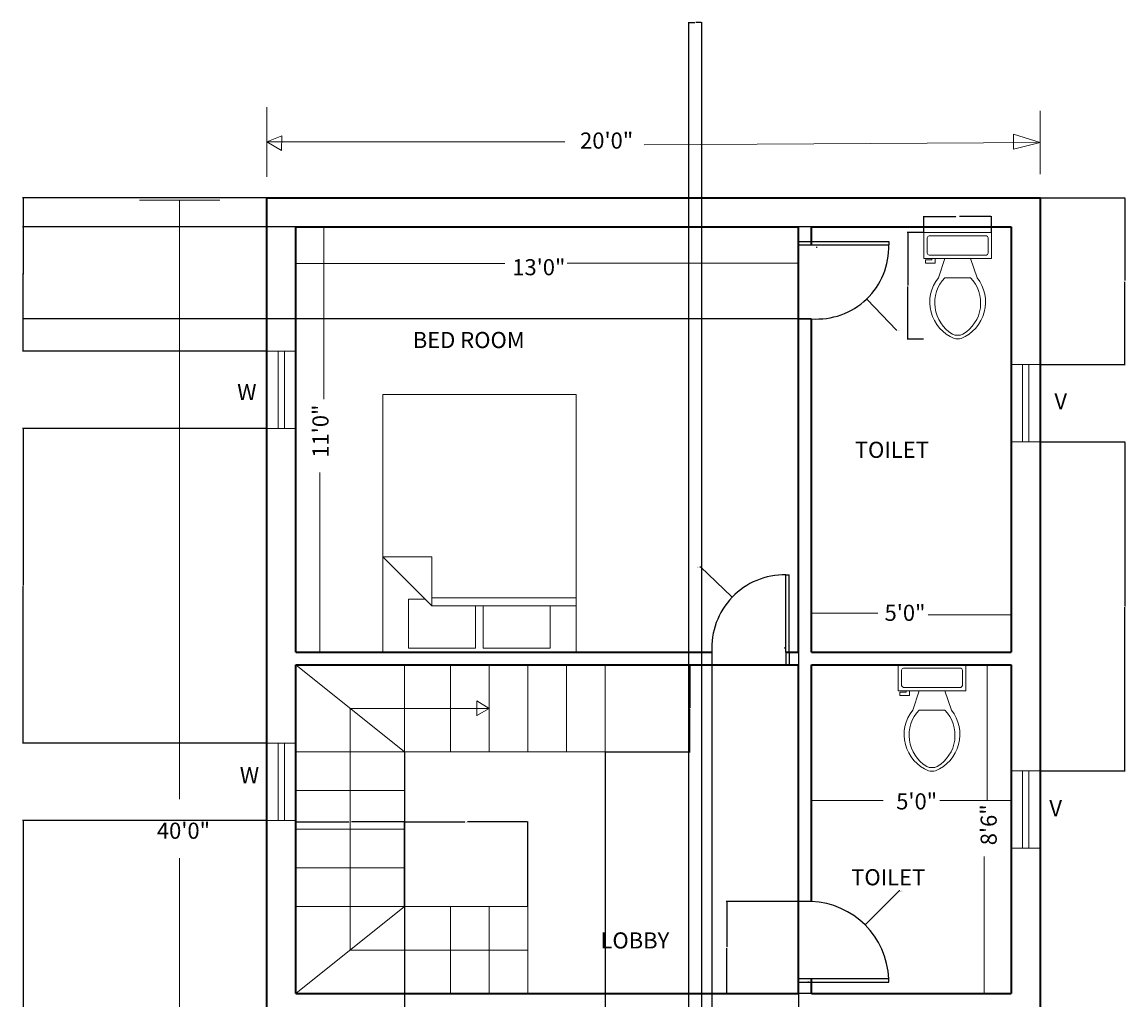
# Model space of a CAD drawing. Units: inches. Extents: x -58 to 719, y -488 to 73.
# Tile 2 of 3: x -58 to 284, y -231 to 73. Entities that reach past the tile are written whole.
import ezdxf

# ---------------------------------------------------------------- set-up
doc = ezdxf.new("R2010")
doc.units = ezdxf.units.IN
doc.header["$MEASUREMENT"] = 0
for name, color, linetype, lineweight in [('A-ANNO-DIMS', 2, 'Continuous', 13), ('A-ANNO-TEXT', 7, 'Continuous', 18), ('A-AREA-IDEN', 7, 'Continuous', 25), ('A-DOOR', 3, 'Continuous', 25), ('A-FLOR-FIXT', 9, 'Continuous', 18), ('A-FLOR-STRS', 7, 'Continuous', 18), ('A-FURN', 8, 'Continuous', 18), ('A-GLAZ', 4, 'Continuous', 18), ('A-WALL', 7, 'Continuous', 35)]:
    doc.layers.add(name, color=color, linetype=linetype, lineweight=lineweight)
doc.styles.get("Standard").update_dxf_attribs({"font": 'arial.ttf'})
doc.dimstyles.get("Standard").update_dxf_attribs({"dimtxt": 0.18, "dimasz": 0.18, "dimexe": 0.18, "dimexo": 0.0625, "dimgap": 0.09, "dimtad": 0, "dimtih": 1, "dimtoh": 1, "dimdec": 4, "dimzin": 0, "dimdsep": 46, "dimtxsty": 'Standard', "dimcen": 0.09, "dimadec": 0, "dimazin": 0, "dimtfac": 1, "dimtdec": 4, "dimtofl": 0, "dimtmove": 0, "dimatfit": 3, "dimfxl": 1, "dimtolj": 1, "dimtzin": 0, "dimarcsym": 0})

# ---------------------------------------------------------------- blocks, each defined once
blk = doc.blocks.new('Bed - Queen')
for p, q in [((0, -80.00003), (0, 0)), ((0, 0), (59.99999, 0)), ((59.99999, 0), (59.99999, -80.00003)), ((7.99999, -1.2), (28.79998, -1.2)), ((7.99999, -14.4), (7.99999, -1.2)), ((28.79998, -1.2), (28.79998, -14.4)), ((31.19999, -1.2), (51.99999, -1.2)), ((31.19999, -14.4), (31.19999, -1.2)), ((51.99999, -1.2), (51.99999, -16.4)), ((0, -14.4), (44.8, -14.4)), ((44.8, -16.8), (0, -16.8)), ((59.99999, -29.6), (44.8, -14.4)), ((44.8, -14.4), (44.8, -29.6)), ((51.99999, -16.4), (46.79936, -16.4)), ((44.8, -29.6), (59.99999, -29.6)), ((59.99999, -80.00003), (0, -80.00003))]:
    blk.add_line(p, q)
blk = doc.blocks.new('Toilet - top')
for p, q in [((9.5, -6), (9.5, -2)), ((-10, -8.5), (-8, -8.5)), ((-10, -9.5), (-10, -8.5)), ((-7, -9.5), (-10, -9.5)), ((-8, -8.5), (-8, -8)), ((-7, -8), (-7, -9.5)), ((-4, -8), (-6, -14)), ((4, -8), (6, -14)), ((4, -14), (-4, -14))]:
    blk.add_line(p, q)
blk.add_lwpolyline([(10.5, -8), (10.5, 0), (-10.5, 0), (-10.5, -8)], close=True)
for points in [[(-9.5, -2), (-9.5, -6)], [(8.5, -1), (-8.5, -1)], [(-8.5, -7), (8.5, -7)]]:
    blk.add_lwpolyline(points)
for centre, radius, start, end in [((-8.62, -1.88), 0.884, 81.8699, 188.1301), ((8.62, -1.88), 0.884, 351.8699, 98.1301), ((-8.62, -6.12), 0.884, 171.8699, 278.1301), ((8.62, -6.12), 0.884, 261.8699, 8.1301), ((3.52, -21.58), 12.17, 141.4691, 247.9714), ((4.2, -21.82), 11.33, 136.3677, 238.9468), ((-3.52, -21.58), 12.17, 292.0284, 38.5307), ((-4.2, -21.82), 11.33, 301.053, 43.6321), ((0, -27.88), 4, 245.7318, 294.2682), ((0, -29), 4, 254.8605, 285.1395)]:
    blk.add_arc(centre, radius, start, end)
blk = doc.blocks.new('WIN-24IN')
for p, q in [((3.5, 24), (3.5, 0)), ((5.5, 24), (5.5, 0))]:
    blk.add_line(p, q)
blk.add_lwpolyline([(0, 24), (9, 24), (9, 0), (0, 0)], close=True)
blk = doc.blocks.new('VENT-24IN')
for p, q in [((3.5, 24), (3.5, 0)), ((5.5, 24), (5.5, 0))]:
    blk.add_line(p, q)
blk.add_lwpolyline([(0, 24), (9, 24), (9, 0), (0, 0)], close=True)
blk = doc.blocks.new('*D13')
at = {"layer": 'A-ANNO-DIMS', "color": 0, "lineweight": -2, "transparency": 16777216}
for p, q in [((221.46, 7.7), (216.39, 7.7)), ((216.57, 7.52), (216.57, -8.64)), ((216.57, -25.17), (216.57, -9.01)), ((221.46, -25.35), (216.39, -25.35))]:
    blk.add_line(p, q, dxfattribs=at)
at = {"layer": 'A-ANNO-DIMS', "color": 0, "transparency": 16777216}
for points in [[(216.54, 7.52), (216.6, 7.52), (216.57, 7.7)], [(216.54, -25.17), (216.6, -25.17), (216.57, -25.35)]]:
    blk.add_solid(points, dxfattribs=at)
at = {"layer": 'Defpoints', "color": 0, "transparency": 16777216}
for p in [(216.57, 7.7), (221.53, 7.7), (221.53, -25.35)]:
    blk.add_point(p, dxfattribs=at)
at = {"layer": 'A-ANNO-DIMS', "color": 0, "transparency": 16777216, "insert": (216.57, -8.83), "char_height": 0.18, "attachment_point": 5}
blk.add_mtext('\\A1;WC 33 TYP.', dxfattribs=at)
blk = doc.blocks.new('*D14')
at = {"layer": 'A-ANNO-DIMS', "color": 0, "lineweight": -2, "transparency": 16777216}
for p, q in [((221.53, 7.76), (221.53, 12.83)), ((221.71, 12.65), (231.5, 12.65)), ((242.35, 12.65), (232.56, 12.65)), ((242.53, 7.76), (242.53, 12.83))]:
    blk.add_line(p, q, dxfattribs=at)
at = {"layer": 'A-ANNO-DIMS', "color": 0, "transparency": 16777216}
for points in [[(221.71, 12.68), (221.71, 12.62), (221.53, 12.65)], [(242.35, 12.68), (242.35, 12.62), (242.53, 12.65)]]:
    blk.add_solid(points, dxfattribs=at)
at = {"layer": 'Defpoints', "color": 0, "transparency": 16777216}
for p in [(242.53, 12.65), (221.53, 7.7), (242.53, 7.7)]:
    blk.add_point(p, dxfattribs=at)
at = {"layer": 'A-ANNO-DIMS', "color": 0, "transparency": 16777216, "insert": (232.03, 12.65), "char_height": 0.18, "attachment_point": 5}
blk.add_mtext('\\A1;21 TYP.', dxfattribs=at)
blk = doc.blocks.new('*D28')
at = {"layer": 'A-ANNO-DIMS', "color": 0, "lineweight": -2, "transparency": 16777216}
for p, q in [((17.55, 18.48), (-58.2, 18.48)), ((-58.02, 18.3), (-58.02, -5.15)), ((-58.02, -28.97), (-58.02, -5.52)), ((17.55, -29.15), (-58.2, -29.15))]:
    blk.add_line(p, q, dxfattribs=at)
at = {"layer": 'A-ANNO-DIMS', "color": 0, "transparency": 16777216}
for points in [[(-58.05, 18.3), (-57.99, 18.3), (-58.02, 18.48)], [(-58.05, -28.97), (-57.99, -28.97), (-58.02, -29.15)]]:
    blk.add_solid(points, dxfattribs=at)
at = {"layer": 'Defpoints', "color": 0, "transparency": 16777216}
for p in [(17.61, 18.48), (-58.02, -29.15), (17.61, -29.15)]:
    blk.add_point(p, dxfattribs=at)
at = {"layer": 'A-ANNO-DIMS', "color": 0, "transparency": 16777216, "insert": (-58.02, -5.34), "char_height": 0.18, "attachment_point": 5}
blk.add_mtext('\\A1;47.63', dxfattribs=at)
blk = doc.blocks.new('*D29')
at = {"layer": 'A-ANNO-DIMS', "color": 0, "lineweight": -2, "transparency": 16777216}
for p, q in [((17.55, -53.15), (-58.2, -53.15)), ((-58.02, -53.33), (-58.02, -101.81)), ((-58.02, -150.65), (-58.02, -102.17)), ((17.55, -150.83), (-58.2, -150.83))]:
    blk.add_line(p, q, dxfattribs=at)
at = {"layer": 'A-ANNO-DIMS', "color": 0, "transparency": 16777216}
for points in [[(-58.05, -53.33), (-57.99, -53.33), (-58.02, -53.15)], [(-58.05, -150.65), (-57.99, -150.65), (-58.02, -150.83)]]:
    blk.add_solid(points, dxfattribs=at)
at = {"layer": 'Defpoints', "color": 0, "transparency": 16777216}
for p in [(17.61, -53.15), (-58.02, -150.83), (17.61, -150.83)]:
    blk.add_point(p, dxfattribs=at)
at = {"layer": 'A-ANNO-DIMS', "color": 0, "transparency": 16777216, "insert": (-58.02, -101.99), "char_height": 0.18, "attachment_point": 5}
blk.add_mtext('\\A1;97.68', dxfattribs=at)
blk = doc.blocks.new('*D30')
at = {"layer": 'A-ANNO-DIMS', "color": 0, "lineweight": -2, "transparency": 16777216}
for p, q in [((17.55, -174.83), (-58.2, -174.83)), ((-58.02, -175.01), (-58.02, -256.1)), ((-58.02, -337.55), (-58.02, -256.46)), ((17.55, -337.73), (-58.2, -337.73))]:
    blk.add_line(p, q, dxfattribs=at)
at = {"layer": 'A-ANNO-DIMS', "color": 0, "transparency": 16777216}
for points in [[(-58.05, -175.01), (-57.99, -175.01), (-58.02, -174.83)], [(-58.05, -337.55), (-57.99, -337.55), (-58.02, -337.73)]]:
    blk.add_solid(points, dxfattribs=at)
at = {"layer": 'Defpoints', "color": 0, "transparency": 16777216}
for p in [(17.61, -174.83), (-58.02, -337.73), (17.61, -337.73)]:
    blk.add_point(p, dxfattribs=at)
at = {"layer": 'A-ANNO-DIMS', "color": 0, "transparency": 16777216, "insert": (-58.02, -256.28), "char_height": 0.18, "attachment_point": 5}
blk.add_mtext('\\A1;162.9', dxfattribs=at)
blk = doc.blocks.new('*D31')
at = {"layer": 'A-ANNO-DIMS', "color": 0, "lineweight": -2, "transparency": 16777216}
for p, q in [((257.67, 18.48), (284.04, 18.48)), ((283.86, 18.3), (283.86, -7.21)), ((283.86, -33.08), (283.86, -7.57)), ((257.67, -33.26), (284.04, -33.26))]:
    blk.add_line(p, q, dxfattribs=at)
at = {"layer": 'A-ANNO-DIMS', "color": 0, "transparency": 16777216}
for points in [[(283.83, 18.3), (283.89, 18.3), (283.86, 18.48)], [(283.83, -33.08), (283.89, -33.08), (283.86, -33.26)]]:
    blk.add_solid(points, dxfattribs=at)
at = {"layer": 'Defpoints', "color": 0, "transparency": 16777216}
for p in [(257.61, 18.48), (257.61, -33.26), (283.86, -33.26)]:
    blk.add_point(p, dxfattribs=at)
at = {"layer": 'A-ANNO-DIMS', "color": 0, "transparency": 16777216, "insert": (283.86, -7.39), "char_height": 0.18, "attachment_point": 5}
blk.add_mtext('\\A1;51.74', dxfattribs=at)
blk = doc.blocks.new('*D32')
at = {"layer": 'A-ANNO-DIMS', "color": 0, "lineweight": -2, "transparency": 16777216}
for p, q in [((257.67, -57.26), (284.04, -57.26)), ((283.86, -57.44), (283.86, -108.16)), ((283.86, -159.24), (283.86, -108.52)), ((257.67, -159.42), (284.04, -159.42))]:
    blk.add_line(p, q, dxfattribs=at)
at = {"layer": 'A-ANNO-DIMS', "color": 0, "transparency": 16777216}
for points in [[(283.83, -57.44), (283.89, -57.44), (283.86, -57.26)], [(283.83, -159.24), (283.89, -159.24), (283.86, -159.42)]]:
    blk.add_solid(points, dxfattribs=at)
at = {"layer": 'Defpoints', "color": 0, "transparency": 16777216}
for p in [(257.61, -57.26), (257.61, -159.42), (283.86, -159.42)]:
    blk.add_point(p, dxfattribs=at)
at = {"layer": 'A-ANNO-DIMS', "color": 0, "transparency": 16777216, "insert": (283.86, -108.34), "char_height": 0.18, "attachment_point": 5}
blk.add_mtext('\\A1;102.16', dxfattribs=at)
blk = doc.blocks.new('*D41')
at = {"layer": 'A-ANNO-DIMS', "color": 0, "lineweight": -2, "transparency": 16777216}
for p, q in [((26.61, -201.46), (26.61, -175.09)), ((26.79, -175.27), (43.1, -175.27)), ((60.2, -175.27), (43.89, -175.27)), ((60.38, -201.46), (60.38, -175.09))]:
    blk.add_line(p, q, dxfattribs=at)
at = {"layer": 'A-ANNO-DIMS', "color": 0, "transparency": 16777216}
for points in [[(26.79, -175.24), (26.79, -175.3), (26.61, -175.27)], [(60.2, -175.24), (60.2, -175.3), (60.38, -175.27)]]:
    blk.add_solid(points, dxfattribs=at)
at = {"layer": 'Defpoints', "color": 0, "transparency": 16777216}
for p in [(60.38, -175.27), (26.61, -201.52), (60.38, -201.52)]:
    blk.add_point(p, dxfattribs=at)
at = {"layer": 'A-ANNO-DIMS', "color": 0, "transparency": 16777216, "insert": (43.5, -175.27), "char_height": 0.18, "attachment_point": 5}
blk.add_mtext('\\A1;33.77', dxfattribs=at)
blk = doc.blocks.new('*D42')
at = {"layer": 'A-ANNO-DIMS', "color": 0, "lineweight": -2, "transparency": 16777216}
for p, q in [((122.67, -126.52), (149.04, -126.52)), ((148.86, -126.7), (148.86, -139.84)), ((148.86, -153.34), (148.86, -140.2)), ((122.67, -153.52), (149.04, -153.52))]:
    blk.add_line(p, q, dxfattribs=at)
at = {"layer": 'A-ANNO-DIMS', "color": 0, "transparency": 16777216}
for points in [[(148.83, -126.7), (148.89, -126.7), (148.86, -126.52)], [(148.83, -153.34), (148.89, -153.34), (148.86, -153.52)]]:
    blk.add_solid(points, dxfattribs=at)
at = {"layer": 'Defpoints', "color": 0, "transparency": 16777216}
for p in [(122.61, -126.52), (122.61, -153.52), (148.86, -153.52)]:
    blk.add_point(p, dxfattribs=at)
at = {"layer": 'A-ANNO-DIMS', "color": 0, "transparency": 16777216, "insert": (148.86, -140.02), "char_height": 0.18, "attachment_point": 5}
blk.add_mtext('\\A1;27', dxfattribs=at)
blk = doc.blocks.new('*D43')
at = {"layer": 'A-ANNO-DIMS', "color": 0, "lineweight": -2, "transparency": 16777216}
for p, q in [((60.38, -153.59), (60.38, -487.95)), ((122.61, -153.59), (122.61, -487.95)), ((60.56, -487.77), (91.1, -487.77)), ((122.43, -487.77), (91.89, -487.77))]:
    blk.add_line(p, q, dxfattribs=at)
at = {"layer": 'A-ANNO-DIMS', "color": 0, "transparency": 16777216}
for points in [[(60.56, -487.74), (60.56, -487.8), (60.38, -487.77)], [(122.43, -487.74), (122.43, -487.8), (122.61, -487.77)]]:
    blk.add_solid(points, dxfattribs=at)
at = {"layer": 'Defpoints', "color": 0, "transparency": 16777216}
for p in [(60.38, -153.52), (122.61, -153.52), (122.61, -487.77)]:
    blk.add_point(p, dxfattribs=at)
at = {"layer": 'A-ANNO-DIMS', "color": 0, "transparency": 16777216, "insert": (91.5, -487.77), "char_height": 0.18, "attachment_point": 5}
blk.add_mtext('\\A1;62.23', dxfattribs=at)
blk = doc.blocks.new('*D44')
at = {"layer": 'A-ANNO-DIMS', "color": 0, "lineweight": -2, "transparency": 16777216}
for p, q in [((60.38, -201.46), (60.38, -175.09)), ((60.56, -175.27), (79.1, -175.27)), ((98.43, -175.27), (79.89, -175.27)), ((98.61, -201.46), (98.61, -175.09))]:
    blk.add_line(p, q, dxfattribs=at)
at = {"layer": 'A-ANNO-DIMS', "color": 0, "transparency": 16777216}
for points in [[(60.56, -175.24), (60.56, -175.3), (60.38, -175.27)], [(98.43, -175.24), (98.43, -175.3), (98.61, -175.27)]]:
    blk.add_solid(points, dxfattribs=at)
at = {"layer": 'Defpoints', "color": 0, "transparency": 16777216}
for p in [(98.61, -175.27), (60.38, -201.52), (98.61, -201.52)]:
    blk.add_point(p, dxfattribs=at)
at = {"layer": 'A-ANNO-DIMS', "color": 0, "transparency": 16777216, "insert": (79.5, -175.27), "char_height": 0.18, "attachment_point": 5}
blk.add_mtext('\\A1;38.23', dxfattribs=at)
blk = doc.blocks.new('*D49')
at = {"layer": 'A-ANNO-DIMS', "color": 0, "lineweight": -2, "transparency": 16777216}
for p, q in [((155.75, -122.59), (155.75, -487.95)), ((182.61, -122.59), (182.61, -487.95)), ((155.93, -487.77), (168.71, -487.77)), ((182.43, -487.77), (169.64, -487.77))]:
    blk.add_line(p, q, dxfattribs=at)
at = {"layer": 'A-ANNO-DIMS', "color": 0, "transparency": 16777216}
for points in [[(155.93, -487.74), (155.93, -487.8), (155.75, -487.77)], [(182.43, -487.74), (182.43, -487.8), (182.61, -487.77)]]:
    blk.add_solid(points, dxfattribs=at)
at = {"layer": 'Defpoints', "color": 0, "transparency": 16777216}
for p in [(155.75, -122.52), (182.61, -122.52), (182.61, -487.77)]:
    blk.add_point(p, dxfattribs=at)
at = {"layer": 'A-ANNO-DIMS', "color": 0, "transparency": 16777216, "insert": (169.18, -487.77), "char_height": 0.18, "attachment_point": 5}
blk.add_mtext('\\A1;26.867', dxfattribs=at)
blk = doc.blocks.new('*D50')
at = {"layer": 'A-ANNO-DIMS', "color": 0, "lineweight": -2, "transparency": 16777216}
for p, q in [((186.55, 9.48), (-58.2, 9.48)), ((-58.02, 9.3), (-58.02, -4.61)), ((-58.02, -18.88), (-58.02, -4.98)), ((186.55, -19.06), (-58.2, -19.06))]:
    blk.add_line(p, q, dxfattribs=at)
at = {"layer": 'A-ANNO-DIMS', "color": 0, "transparency": 16777216}
for points in [[(-58.05, 9.3), (-57.99, 9.3), (-58.02, 9.48)], [(-58.05, -18.88), (-57.99, -18.88), (-58.02, -19.06)]]:
    blk.add_solid(points, dxfattribs=at)
at = {"layer": 'Defpoints', "color": 0, "transparency": 16777216}
for p in [(186.61, 9.48), (-58.02, -19.06), (186.61, -19.06)]:
    blk.add_point(p, dxfattribs=at)
at = {"layer": 'A-ANNO-DIMS', "color": 0, "transparency": 16777216, "insert": (-58.02, -4.79), "char_height": 0.18, "attachment_point": 5}
blk.add_mtext('\\A1;28.54', dxfattribs=at)
blk = doc.blocks.new('*D51')
at = {"layer": 'A-ANNO-DIMS', "color": 0, "lineweight": -2, "transparency": 16777216}
for p, q in [((186.55, -199.98), (160.18, -199.98)), ((160.36, -200.16), (160.36, -214.07)), ((160.36, -228.34), (160.36, -214.43)), ((186.55, -228.52), (160.18, -228.52))]:
    blk.add_line(p, q, dxfattribs=at)
at = {"layer": 'A-ANNO-DIMS', "color": 0, "transparency": 16777216}
for points in [[(160.33, -200.16), (160.39, -200.16), (160.36, -199.98)], [(160.33, -228.34), (160.39, -228.34), (160.36, -228.52)]]:
    blk.add_solid(points, dxfattribs=at)
at = {"layer": 'Defpoints', "color": 0, "transparency": 16777216}
for p in [(160.36, -199.98), (186.61, -199.98), (186.61, -228.52)]:
    blk.add_point(p, dxfattribs=at)
at = {"layer": 'A-ANNO-DIMS', "color": 0, "transparency": 16777216, "insert": (160.36, -214.25), "char_height": 0.18, "attachment_point": 5}
blk.add_mtext('\\A1;28.54', dxfattribs=at)
blk = doc.blocks.new('*D57')
at = {"layer": 'A-ANNO-DIMS', "color": 0, "lineweight": -2, "transparency": 16777216}
for p, q in [((148.61, -377.52), (148.61, 73.06)), ((148.79, 72.88), (150.46, 72.88)), ((152.43, 72.88), (150.76, 72.88)), ((152.61, -377.52), (152.61, 73.06))]:
    blk.add_line(p, q, dxfattribs=at)
at = {"layer": 'A-ANNO-DIMS', "color": 0, "transparency": 16777216}
for points in [[(148.79, 72.91), (148.79, 72.85), (148.61, 72.88)], [(152.43, 72.91), (152.43, 72.85), (152.61, 72.88)]]:
    blk.add_solid(points, dxfattribs=at)
at = {"layer": 'Defpoints', "color": 0, "transparency": 16777216}
for p in [(152.61, 72.88), (148.61, -377.58), (152.61, -377.58)]:
    blk.add_point(p, dxfattribs=at)
at = {"layer": 'A-ANNO-DIMS', "color": 0, "transparency": 16777216, "insert": (150.61, 72.88), "char_height": 0.18, "attachment_point": 5}
blk.add_mtext('\\A1;4', dxfattribs=at)
blk = doc.blocks.new('*D60')
at = {"layer": 'A-ANNO-DIMS', "color": 0, "lineweight": -2, "transparency": 16777216}
for p, q in [((152, -96.09), (152.18, -96.09)), ((152.18, -96.09), (161.89, -105.39)), ((178.33, -121.23), (178.51, -121.23)), ((178.42, -121.32), (178.42, -121.14))]:
    blk.add_line(p, q, dxfattribs=at)
at = {"layer": 'A-ANNO-DIMS', "color": 0, "transparency": 16777216}
blk.add_solid([(161.91, -105.37), (161.87, -105.41), (162.02, -105.52)], dxfattribs=at)
at = {"layer": 'Defpoints', "color": 0, "transparency": 16777216}
for p in [(162.02, -105.52), (178.42, -121.23)]:
    blk.add_point(p, dxfattribs=at)
at = {"layer": 'A-ANNO-DIMS', "color": 0, "transparency": 16777216, "insert": (151.54, -96.09), "char_height": 0.18, "attachment_point": 5}
blk.add_mtext('\\A1;R22.71', dxfattribs=at)
blk = doc.blocks.new('*D61')
at = {"layer": 'A-ANNO-DIMS', "color": 0, "lineweight": -2, "transparency": 16777216}
for p, q in [((188.26, 3.14), (188.44, 3.14)), ((188.35, 3.05), (188.35, 3.23)), ((213.01, -22.59), (203.89, -13.07)), ((213.19, -22.59), (213.01, -22.59))]:
    blk.add_line(p, q, dxfattribs=at)
at = {"layer": 'A-ANNO-DIMS', "color": 0, "transparency": 16777216}
blk.add_solid([(203.91, -13.05), (203.87, -13.09), (203.77, -12.94)], dxfattribs=at)
at = {"layer": 'Defpoints', "color": 0, "transparency": 16777216}
for p in [(188.35, 3.14), (203.77, -12.94)]:
    blk.add_point(p, dxfattribs=at)
at = {"layer": 'A-ANNO-DIMS', "color": 0, "transparency": 16777216, "insert": (213.74, -22.59), "char_height": 0.18, "attachment_point": 5}
blk.add_mtext('\\A1;R22.273', dxfattribs=at)
blk = doc.blocks.new('*D62')
at = {"layer": 'A-ANNO-DIMS', "color": 0, "lineweight": -2, "transparency": 16777216}
for p, q in [((213.9, -196.7), (203.46, -207.13)), ((214.08, -196.7), (213.9, -196.7)), ((185.65, -224.86), (185.83, -224.86)), ((185.74, -224.95), (185.74, -224.77))]:
    blk.add_line(p, q, dxfattribs=at)
at = {"layer": 'A-ANNO-DIMS', "color": 0, "transparency": 16777216}
blk.add_solid([(203.44, -207.11), (203.49, -207.15), (203.34, -207.26)], dxfattribs=at)
at = {"layer": 'Defpoints', "color": 0, "transparency": 16777216}
for p in [(203.34, -207.26), (185.74, -224.86)]:
    blk.add_point(p, dxfattribs=at)
at = {"layer": 'A-ANNO-DIMS', "color": 0, "transparency": 16777216, "insert": (214.56, -196.7), "char_height": 0.18, "attachment_point": 5}
blk.add_mtext('\\A1;R24.89', dxfattribs=at)

msp = doc.modelspace()

# ---------------------------------------------------------------- linework, layer by layer
at = {"layer": 'A-ANNO-DIMS'}
for p, q in [((17.6125, 25.0283), (17.6125, 46.6293)), ((257.6125, 25.8138), (257.6125, 45.4511)), ((22.2716, 37.7231), (17.6125, 35.8288)), ((22.2315, 33.162), (22.2716, 37.7231)), ((249.366, 38.2807), (249.366, 33.5899)), ((257.6125, 35.6324), (249.366, 38.2807)), ((17.6125, 35.8288), (110.1276, 35.8288)), ((17.6125, 35.8288), (22.2315, 33.162)), ((134.7642, 34.9502), (257.6125, 35.6324)), ((249.366, 33.5899), (257.6125, 35.6324)), ((3.0105, 17.8018), (-21.9117, 17.8018)), ((-9.4506, 17.8018), (-9.4506, -151.1187)), ((35.2818, 9.477), (35.2818, -43.9909)), ((26.6125, -1.9438), (91.5244, -1.9438)), ((110.8063, -1.8001), (182.6125, -1.8001)), ((34.1307, -66.8274), (34.1307, -122.523)), ((207.2932, -110.4277), (186.6125, -110.4277)), ((222.8264, -111.0077), (248.6125, -111.0077)), ((241.1751, -168.631), (241.1751, -126.523)), ((-9.4506, -151.1187), (-9.4506, -168.1887)), ((208.8765, -168.631), (186.6125, -168.631)), ((226.472, -168.631), (248.6125, -168.631)), ((-9.4506, -208.4652), (-9.4506, -186.5319)), ((240.211, -185.9652), (240.211, -228.523)), ((-9.4506, -208.4652), (-9.4506, -461.523))]:
    msp.add_line(p, q, dxfattribs=at)
at = {"layer": 'A-DOOR'}
for p, q in [((182.6125, 4.9358), (186.6125, 4.9358)), ((182.6125, 3.9358), (186.6125, 3.9358)), ((186.6125, 4.9358), (210.6125, 4.9358)), ((186.6125, 3.9358), (210.6125, 3.9358)), ((210.6125, 4.9358), (210.6125, 3.9358)), ((182.6125, -19.0642), (186.6125, -19.0642)), ((178.7455, -122.523), (178.7455, -98.523)), ((178.7455, -98.523), (179.7455, -98.523)), ((179.7455, -122.523), (179.7455, -98.523)), ((155.7455, -122.523), (155.7455, -126.523)), ((178.7455, -122.523), (178.7455, -126.523)), ((179.7455, -122.523), (179.7455, -126.523)), ((186.6125, -199.9829), (182.6125, -199.9829)), ((210.6125, -223.9829), (182.6125, -223.9829)), ((182.6125, -224.9829), (186.6125, -224.9829)), ((186.6125, -224.9829), (210.6125, -224.9829)), ((210.6125, -224.9829), (210.6125, -223.9829))]:
    msp.add_line(p, q, dxfattribs=at)
for centre, radius, start, end in [((188.3542, 3.1401), 22.2725, 265.5149, 2.047349), ((178.42, -121.2319), 22.7112, 89.17876, 183.25899), ((185.7369, -224.8584), 24.891, 2.01582, 87.98418)]:
    msp.add_arc(centre, radius, start, end, dxfattribs=at)
at = {"layer": 'A-FLOR-STRS'}
for p, q in [((26.6125, -126.523), (60.3821, -153.523)), ((60.3821, -126.523), (60.3821, -228.523)), ((74.6125, -153.523), (74.6125, -126.523)), ((86.6125, -153.523), (86.6125, -126.523)), ((98.6125, -153.523), (98.6125, -126.523)), ((110.6125, -153.523), (110.6125, -126.523)), ((122.6125, -153.523), (122.6125, -126.523)), ((43.4973, -215.023), (43.4973, -140.023)), ((43.4973, -140.023), (86.6125, -140.023)), ((82.8428, -137.6838), (82.8428, -142.2823)), ((82.8428, -137.6838), (86.6125, -140.023)), ((86.6125, -140.023), (82.8428, -142.1994)), ((122.6125, -153.523), (26.6125, -153.523)), ((60.3821, -165.523), (26.6125, -165.523)), ((60.3821, -177.523), (26.6125, -177.523)), ((60.3821, -189.523), (26.6125, -189.523)), ((98.6125, -201.523), (26.6125, -201.523)), ((26.6125, -228.523), (60.3821, -201.523)), ((74.6125, -228.523), (74.6125, -201.523)), ((86.6125, -228.523), (86.6125, -201.523)), ((98.6125, -228.523), (98.6125, -201.523)), ((98.6125, -215.023), (43.4973, -215.023))]:
    msp.add_line(p, q, dxfattribs=at)
at = {"layer": 'A-WALL'}
for p, q in [((26.6125, 9.477), (182.6125, 9.477)), ((26.6125, -122.523), (26.6125, 9.477)), ((182.6125, -122.523), (182.6125, 9.477)), ((186.6125, 9.477), (248.6125, 9.477)), ((186.6125, 3.9358), (186.6125, 9.477)), ((248.6125, 9.477), (248.6125, -122.523)), ((186.6125, -122.523), (186.6125, -19.0642)), ((26.6125, -122.523), (155.7455, -122.523)), ((178.7455, -122.523), (182.6125, -122.523)), ((186.6125, -122.523), (248.6125, -122.523)), ((26.6125, -126.523), (182.6125, -126.523)), ((26.6125, -228.523), (26.6125, -126.523)), ((182.6125, -228.523), (182.6125, -126.523)), ((186.6125, -126.523), (248.6125, -126.523)), ((186.6125, -199.9829), (186.6125, -126.523)), ((248.6125, -126.523), (248.6125, -228.523)), ((186.6125, -228.523), (186.6125, -223.9829)), ((26.6125, -228.523), (182.6125, -228.523)), ((186.6125, -228.523), (248.6125, -228.523))]:
    msp.add_line(p, q, dxfattribs=at)
msp.add_lwpolyline([(17.6125, 18.477), (257.6125, 18.477), (257.6125, -461.523), (17.6125, -461.523)], close=True, dxfattribs=at)

# ---------------------------------------------------------------- block references
at = {"layer": 'A-FLOR-FIXT'}
for p in [(232.0273, 7.6958), (224.0617, -126.523)]:
    msp.add_blockref('Toilet - top', p, dxfattribs=at)
at = {"layer": 'A-FURN', "rotation": 180}
msp.add_blockref('Bed - Queen', (113.5937, -122.523), dxfattribs=at)
at = {"layer": 'A-GLAZ'}
for name, p in [('WIN-24IN', (17.612, -53.15)), ('VENT-24IN', (248.612, -57.262)), ('WIN-24IN', (17.612, -174.8327)), ('VENT-24IN', (248.612, -183.419))]:
    msp.add_blockref(name, p, dxfattribs=at)

# ---------------------------------------------------------------- texts
at = {"layer": 'A-ANNO-DIMS', "char_height": 5, "attachment_point": 1}
for s, width, insert in [('20\'0"', 28.703953, (114.8461, 38.7744)), ('13\'0"', 29.490631, (93.7994, -0.5447)), ('5\'0"', 18.491526, (209.3359, -107.8433)), ('5\'0"', 25.867981, (212.953, -166.3822)), ('40\'0"', 31.98226, (-16.4861, -175.484))]:
    msp.add_mtext_dynamic_manual_height_columns(s, width=width, gutter_width=25, heights=[0], dxfattribs=dict(at, insert=insert))
at = {"layer": 'A-ANNO-DIMS', "char_height": 5, "attachment_point": 1, "rotation": 90}
for s, width, insert in [('11\'0"', 10.973264, (31.782, -62.1803)), ('8\'6"', 12.173174, (239.1427, -182.507))]:
    msp.add_mtext_dynamic_manual_height_columns(s, width=width, gutter_width=25, heights=[0], dxfattribs=dict(at, insert=insert))
at = {"layer": 'A-ANNO-TEXT', "char_height": 5, "attachment_point": 1}
for s, width, insert in [('W', 17.81108, (8.4361, -39.3163)), ('V', 10.767555, (262.0349, -42.1619)), ('W', 14.30611, (9.2437, -158.2478)), ('V', 11.337096, (260.4655, -168.4838))]:
    msp.add_mtext_dynamic_manual_height_columns(s, width=width, gutter_width=25, heights=[0], dxfattribs=dict(at, insert=insert))
at = {"layer": 'A-AREA-IDEN', "char_height": 5, "attachment_point": 1}
for s, width, insert in [('BED ROOM', 52.122972, (62.9371, -23.1505)), ('TOILET', 36.88469, (200.1267, -57.2357)), ('TOILET', 33.856624, (198.9865, -189.9401)), ('LOBBY', 41.464849, (121.1802, -209.5542))]:
    msp.add_mtext_dynamic_manual_height_columns(s, width=width, gutter_width=25, heights=[0], dxfattribs=dict(at, insert=insert))

# ---------------------------------------------------------------- dimensions: what is measured, and where the dimension line sits
at = {"layer": 'A-ANNO-DIMS'}
for base, p1, p2, override, picture, middle in [((152.6125, 72.8793), (148.6125, -377.5847), (152.6125, -377.5847), {"dimdec": 0, "dimlfac": 1, "dimrnd": 0, "dimzin": 0, "dimdsep": 46, "dimlunit": 2}, '*D57', (150.6125, 72.8793)), ((182.6125, -487.773), (155.7455, -122.523), (182.6125, -122.523), {"dimdec": 3, "dimlfac": 1, "dimrnd": 0, "dimzin": 0, "dimdsep": 46, "dimlunit": 2}, '*D49', (169.179, -487.773)), ((122.6125, -487.773), (60.3821, -153.523), (122.6125, -153.523), {"dimdec": 2, "dimlfac": 1, "dimrnd": 0, "dimzin": 0, "dimdsep": 46, "dimlunit": 2}, '*D43', (91.4973, -487.773)), ((60.3821, -175.273), (26.6125, -201.523), (60.3821, -201.523), {"dimdec": 2, "dimlfac": 1, "dimrnd": 0, "dimzin": 0, "dimdsep": 46, "dimlunit": 2}, '*D41', (43.4973, -175.273)), ((98.6125, -175.273), (60.3821, -201.523), (98.6125, -201.523), {"dimdec": 2, "dimlfac": 1, "dimrnd": 0, "dimzin": 0, "dimdsep": 46, "dimlunit": 2}, '*D44', (79.4973, -175.273))]:
    dim = msp.add_linear_dim(base=base, p1=p1, p2=p2, dimstyle='Standard', override=override, dxfattribs=at)
    dim.commit()
    dim.dimension.update_dxf_attribs({"geometry": picture, "text_midpoint": middle})
for base, p1, p2, angle, override, picture, middle in [((-58.0187, -29.15), (17.6125, 18.477), (17.6125, -29.15), 90, {"dimdec": 2, "dimlfac": 1, "dimrnd": 0, "dimzin": 0, "dimdsep": 46, "dimlunit": 2}, '*D28', (-58.0187, -5.3365)), ((283.8625, -33.2617), (257.6125, 18.477), (257.6125, -33.2617), 90, {"dimdec": 2, "dimlfac": 1, "dimrnd": 0, "dimzin": 0, "dimdsep": 46, "dimlunit": 2}, '*D31', (283.8625, -7.3923)), ((-58.0187, -19.0642), (186.6125, 9.477), (186.6125, -19.0642), 90, {"dimdec": 2, "dimlfac": 1, "dimrnd": 0, "dimzin": 0, "dimdsep": 46, "dimlunit": 2}, '*D50', (-58.0187, -4.7936)), ((-58.0187, -150.8328), (17.6125, -53.15), (17.6125, -150.8328), 90, {"dimdec": 2, "dimlfac": 1, "dimrnd": 0, "dimzin": 0, "dimdsep": 46, "dimlunit": 2}, '*D29', (-58.0187, -101.9914)), ((283.8625, -159.4187), (257.6125, -57.2617), (257.6125, -159.4187), 90, {"dimdec": 2, "dimlfac": 1, "dimrnd": 0, "dimzin": 0, "dimdsep": 46, "dimlunit": 2}, '*D32', (283.8625, -108.3402)), ((148.8625, -153.523), (122.6125, -126.523), (122.6125, -153.523), 270, {"dimdec": 0, "dimlfac": 1, "dimrnd": 0, "dimzin": 0, "dimdsep": 46, "dimlunit": 2}, '*D42', (148.8625, -140.023)), ((-58.0187, -337.7265), (17.6125, -174.8328), (17.6125, -337.7265), 90, {"dimdec": 1, "dimlfac": 1, "dimrnd": 0, "dimzin": 0, "dimdsep": 46, "dimlunit": 2}, '*D30', (-58.0187, -256.2797)), ((160.3625, -199.9829), (186.6125, -228.523), (186.6125, -199.9829), 90, {"dimdec": 2, "dimlfac": 1, "dimrnd": 0, "dimzin": 0, "dimdsep": 46, "dimlunit": 2}, '*D51', (160.3625, -214.2529))]:
    dim = msp.add_linear_dim(base=base, p1=p1, p2=p2, angle=angle, dimstyle='Standard', override=override, dxfattribs=at)
    dim.commit()
    dim.dimension.update_dxf_attribs({"geometry": picture, "text_midpoint": middle})
dim = msp.add_linear_dim(base=(242.5273, 12.6528), p1=(221.5273, 7.6958), p2=(242.5273, 7.6958), text='<> TYP.', dimstyle='Standard', override={"dimdec": 0, "dimlfac": 1, "dimrnd": 0, "dimzin": 0, "dimdsep": 46, "dimlunit": 2}, dxfattribs=at)
dim.commit()
dim.dimension.update_dxf_attribs({"geometry": '*D14', "text_midpoint": (232.0273, 12.6528)})
dim = msp.add_linear_dim(base=(216.5704, 7.6958), p1=(221.5273, -25.3504), p2=(221.5273, 7.6958), angle=90, text='WC <> TYP.', dimstyle='Standard', override={"dimdec": 0, "dimlfac": 1, "dimrnd": 0, "dimzin": 0, "dimdsep": 46, "dimlunit": 2}, dxfattribs=at)
dim.commit()
dim.dimension.update_dxf_attribs({"geometry": '*D13', "text_midpoint": (216.5704, -8.8273)})
for center, mpoint, override, picture, middle in [((188.35418, 3.14015), (203.765, -12.94), {"dimdec": 3, "dimlfac": 1, "dimrnd": 0, "dimzin": 0, "dimdsep": 46, "dimlunit": 2}, '*D61', (213.74126, -22.58809)), ((178.42, -121.2319), (162.0228, -105.5178), {"dimdec": 2, "dimlfac": 1, "dimrnd": 0, "dimzin": 0, "dimdsep": 46, "dimlunit": 2}, '*D60', (151.542, -96.0893)), ((185.7369, -224.8584), (203.3373, -207.2577), {"dimdec": 2, "dimlfac": 1, "dimrnd": 0, "dimzin": 0, "dimdsep": 46, "dimlunit": 2}, '*D62', (214.5576, -196.6973))]:
    dim = msp.add_radius_dim(center=center, mpoint=mpoint, dimstyle='Standard', override=override, dxfattribs=at)
    dim.commit()
    dim.dimension.update_dxf_attribs({"geometry": picture, "text_midpoint": middle, "dimtype": 164})

doc.saveas('drawing.dxf')
